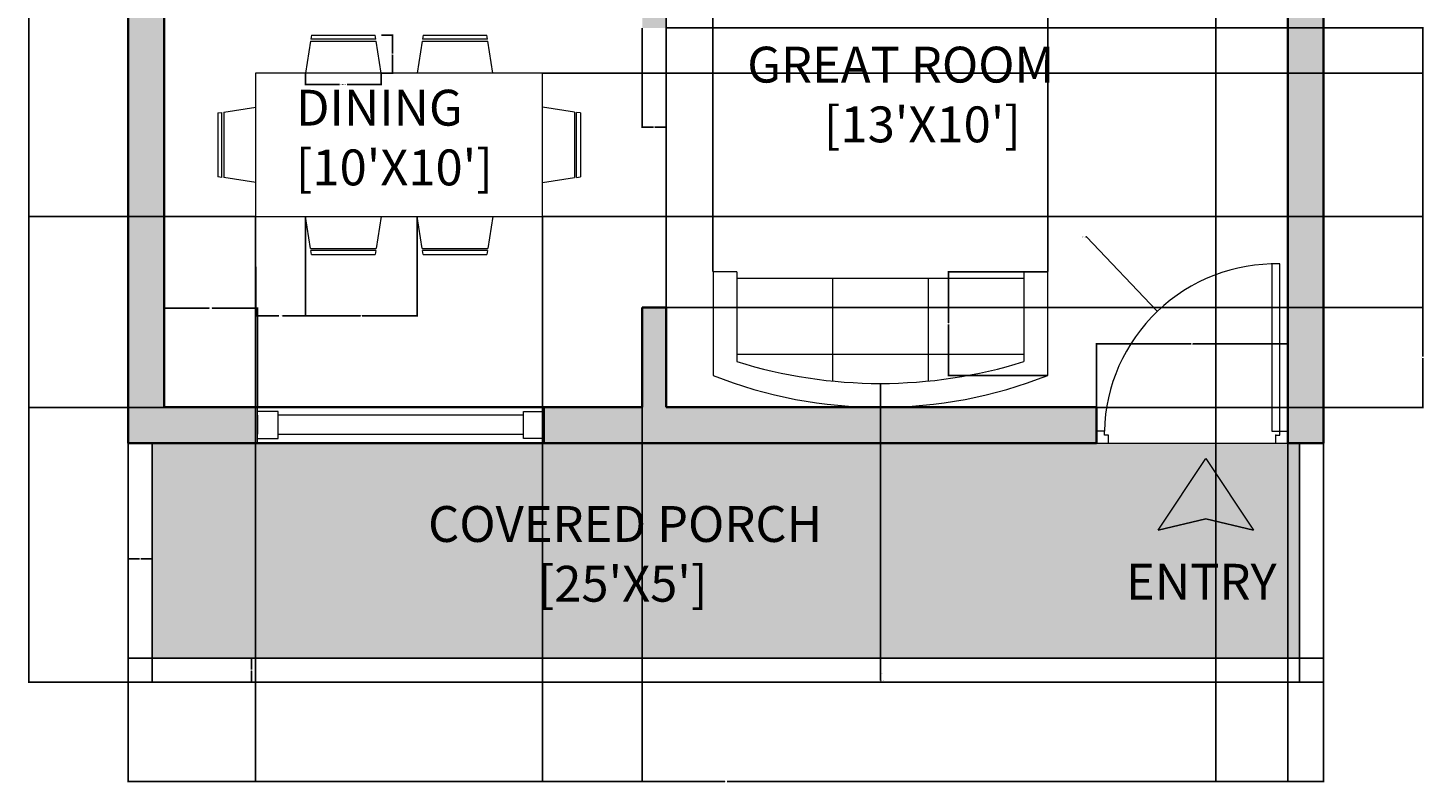
# Model space of a CAD drawing. Units: inches. Extents: x 2203 to 2554, y 381 to 929.
# Tile 1 of 3: x 2203 to 2554, y 381 to 570. Entities that reach past the tile are written whole.
import ezdxf

# ---------------------------------------------------------------- set-up
doc = ezdxf.new("R2010")
doc.units = ezdxf.units.IN
for name, color, linetype, lineweight in [('A-ANNO-DIMS', 2, 'Continuous', 18), ('A-ANNO-SYMB', 239, 'Continuous', 18), ('A-ANNO-TEXT', 7, 'Continuous', 18), ('A-AREA-IDEN', 7, 'Continuous', 18), ('A-DOOR', 239, 'Continuous', 18), ('A-FLOR', 7, 'Continuous', 25), ('A-FURN', 8, 'Continuous', 18), ('A-GLAZ', 4, 'Continuous', 18), ('A-WALL', 7, 'Continuous', 35), ('A-WALL-PATT', 250, 'Continuous', 13)]:
    doc.layers.add(name, color=color, linetype=linetype, lineweight=lineweight)
doc.layers.add('A-FLOR-PATT', color=241, linetype='Continuous', lineweight=13, true_color=0xf7abae)
doc.styles.get("Standard").update_dxf_attribs({"font": 'arial.ttf'})
doc.dimstyles.get("Standard").update_dxf_attribs({"dimtxt": 0.18, "dimasz": 0.18, "dimexe": 0.18, "dimexo": 0.0625, "dimgap": 0.09, "dimtad": 0, "dimtih": 1, "dimtoh": 1, "dimdec": 4, "dimzin": 0, "dimdsep": 46, "dimtxsty": 'Standard', "dimcen": 0.09, "dimadec": 0, "dimazin": 0, "dimtfac": 1, "dimtdec": 4, "dimtofl": 0, "dimtmove": 0, "dimatfit": 3, "dimfxl": 1, "dimtolj": 1, "dimtzin": 0, "dimarcsym": 0})

# ---------------------------------------------------------------- blocks, each defined once
blk = doc.blocks.new('WIN-72')
for p, q in [((0, 0), (0, 9)), ((0, 9), (72, 9)), ((5.2, 7.99), (0, 7.99)), ((5.2, 1.13), (5.2, 7.99)), ((66.8, 1.13), (66.8, 7.99)), ((66.8, 7.99), (72, 7.99)), ((72, 9), (72, 0)), ((72, 6.99), (72, 9)), ((0, 6.99), (0, 2.25)), ((0, 0), (0, 4.5)), ((66.8, 6.99), (5.2, 6.99)), ((72, 4.5), (72, 6.99)), ((72, 2.25), (72, 6.99)), ((0, 1.13), (5.2, 1.13)), ((72, 0), (0, 0)), ((5.2, 2.25), (66.8, 2.25)), ((72, 1.13), (66.8, 1.13)), ((72, 0), (72, 2.25))]:
    blk.add_line(p, q)
blk = doc.blocks.new('CHAIR-DINING')
for p, q in [((1.2504, 8.00297), (0, 0)), ((1.2543, 8.00238), (17.7239, 8.00238)), ((1.4847, 9.50238), (1.3285, 8.5028)), ((17.6431, 8.50238), (1.3313, 8.50238)), ((1.4847, 9.50238), (17.4847, 9.50238)), ((17.641, 8.50204), (17.4847, 9.50238)), ((18.9695, 0), (17.7192, 8.00164))]:
    blk.add_line(p, q)
blk = doc.blocks.new('*D13')
at = {"layer": 'A-ANNO-DIMS', "color": 0, "lineweight": -2, "transparency": 16777216}
for p, q in [((2273.11, 558.9), (2273.11, 555.94)), ((2292.08, 558.9), (2292.08, 555.94)), ((2273.29, 556.12), (2281.64, 556.12)), ((2291.9, 556.12), (2283.55, 556.12))]:
    blk.add_line(p, q, dxfattribs=at)
at = {"layer": 'A-ANNO-DIMS', "color": 0, "transparency": 16777216}
for points in [[(2273.29, 556.15), (2273.29, 556.09), (2273.11, 556.12)], [(2291.9, 556.15), (2291.9, 556.09), (2292.08, 556.12)]]:
    blk.add_solid(points, dxfattribs=at)
at = {"layer": 'Defpoints', "color": 0, "transparency": 16777216}
for p in [(2273.11, 558.96), (2292.08, 558.96), (2292.08, 556.12)]:
    blk.add_point(p, dxfattribs=at)
at = {"layer": 'A-ANNO-DIMS', "color": 0, "transparency": 16777216, "insert": (2282.59, 556.12), "char_height": 0.18, "attachment_point": 5}
blk.add_mtext('\\A1;CHAIR 19 TYP.', dxfattribs=at)
blk = doc.blocks.new('*D14')
at = {"layer": 'A-ANNO-DIMS', "color": 0, "lineweight": -2, "transparency": 16777216}
for p, q in [((2292.14, 568.47), (2295.1, 568.47)), ((2294.92, 568.29), (2294.92, 563.9)), ((2294.92, 559.14), (2294.92, 563.53)), ((2292.14, 558.96), (2295.1, 558.96))]:
    blk.add_line(p, q, dxfattribs=at)
at = {"layer": 'A-ANNO-DIMS', "color": 0, "transparency": 16777216}
for points in [[(2294.89, 568.29), (2294.95, 568.29), (2294.92, 568.47)], [(2294.89, 559.14), (2294.95, 559.14), (2294.92, 558.96)]]:
    blk.add_solid(points, dxfattribs=at)
at = {"layer": 'Defpoints', "color": 0, "transparency": 16777216}
for p in [(2292.08, 568.47), (2294.92, 568.47), (2292.08, 558.96)]:
    blk.add_point(p, dxfattribs=at)
at = {"layer": 'A-ANNO-DIMS', "color": 0, "transparency": 16777216, "insert": (2294.92, 563.71), "char_height": 0.18, "attachment_point": 5}
blk.add_mtext('\\A1;10 TYP.', dxfattribs=at)
blk = doc.blocks.new('*D21')
at = {"layer": 'A-ANNO-DIMS', "color": 0, "lineweight": -2, "transparency": 16777216}
for p, q in [((2228.6, 406), (2228.6, 380.96)), ((2528.6, 406), (2528.6, 380.96)), ((2228.78, 381.14), (2378.31, 381.14)), ((2528.42, 381.14), (2378.89, 381.14))]:
    blk.add_line(p, q, dxfattribs=at)
at = {"layer": 'A-ANNO-DIMS', "color": 0, "transparency": 16777216}
for points in [[(2228.78, 381.17), (2228.78, 381.11), (2228.6, 381.14)], [(2528.42, 381.17), (2528.42, 381.11), (2528.6, 381.14)]]:
    blk.add_solid(points, dxfattribs=at)
at = {"layer": 'Defpoints', "color": 0, "transparency": 16777216}
for p in [(2228.6, 406.06), (2528.6, 406.06), (2528.6, 381.14)]:
    blk.add_point(p, dxfattribs=at)
at = {"layer": 'A-ANNO-DIMS', "color": 0, "transparency": 16777216, "insert": (2378.6, 381.14), "char_height": 0.18, "attachment_point": 5}
blk.add_mtext('\\A1;300', dxfattribs=at)
blk = doc.blocks.new('*D22')
at = {"layer": 'A-ANNO-DIMS', "color": 0, "lineweight": -2, "transparency": 16777216}
for p, q in [((2228.54, 904.06), (2203.5, 904.06)), ((2203.68, 903.88), (2203.68, 655.25)), ((2203.68, 406.24), (2203.68, 654.88)), ((2228.54, 406.06), (2203.5, 406.06))]:
    blk.add_line(p, q, dxfattribs=at)
at = {"layer": 'A-ANNO-DIMS', "color": 0, "transparency": 16777216}
for points in [[(2203.65, 903.88), (2203.71, 903.88), (2203.68, 904.06)], [(2203.65, 406.24), (2203.71, 406.24), (2203.68, 406.06)]]:
    blk.add_solid(points, dxfattribs=at)
at = {"layer": 'Defpoints', "color": 0, "transparency": 16777216}
for p in [(2203.68, 904.06), (2228.6, 904.06), (2228.6, 406.06)]:
    blk.add_point(p, dxfattribs=at)
at = {"layer": 'A-ANNO-DIMS', "color": 0, "transparency": 16777216, "insert": (2203.68, 655.06), "char_height": 0.18, "attachment_point": 5}
blk.add_mtext('\\A1;498', dxfattribs=at)
blk = doc.blocks.new('*D25')
at = {"layer": 'A-ANNO-DIMS', "color": 0, "lineweight": -2, "transparency": 16777216}
for p, q in [((2237.6, 475.13), (2237.6, 500.16)), ((2237.78, 499.98), (2248.92, 499.98)), ((2260.85, 499.98), (2249.71, 499.98)), ((2261.03, 475.13), (2261.03, 500.16))]:
    blk.add_line(p, q, dxfattribs=at)
at = {"layer": 'A-ANNO-DIMS', "color": 0, "transparency": 16777216}
for points in [[(2237.78, 500.01), (2237.78, 499.95), (2237.6, 499.98)], [(2260.85, 500.01), (2260.85, 499.95), (2261.03, 499.98)]]:
    blk.add_solid(points, dxfattribs=at)
at = {"layer": 'Defpoints', "color": 0, "transparency": 16777216}
for p in [(2261.03, 499.98), (2237.6, 475.06), (2261.03, 475.06)]:
    blk.add_point(p, dxfattribs=at)
at = {"layer": 'A-ANNO-DIMS', "color": 0, "transparency": 16777216, "insert": (2249.31, 499.98), "char_height": 0.18, "attachment_point": 5}
blk.add_mtext('\\A1;23.43', dxfattribs=at)
blk = doc.blocks.new('*D28')
at = {"layer": 'A-ANNO-DIMS', "color": 0, "lineweight": -2, "transparency": 16777216}
for p, q in [((2357.6, 570.27), (2357.6, 545.23)), ((2363.6, 570.27), (2363.6, 545.23)), ((2357.78, 545.41), (2360.45, 545.41)), ((2363.42, 545.41), (2360.75, 545.41))]:
    blk.add_line(p, q, dxfattribs=at)
at = {"layer": 'A-ANNO-DIMS', "color": 0, "transparency": 16777216}
for points in [[(2357.78, 545.44), (2357.78, 545.38), (2357.6, 545.41)], [(2363.42, 545.44), (2363.42, 545.38), (2363.6, 545.41)]]:
    blk.add_solid(points, dxfattribs=at)
at = {"layer": 'Defpoints', "color": 0, "transparency": 16777216}
for p in [(2357.6, 570.33), (2363.6, 570.33), (2357.6, 545.41)]:
    blk.add_point(p, dxfattribs=at)
at = {"layer": 'A-ANNO-DIMS', "color": 0, "transparency": 16777216, "insert": (2360.6, 545.41), "char_height": 0.18, "attachment_point": 5}
blk.add_mtext('\\A1;6', dxfattribs=at)
blk = doc.blocks.new('*D32')
at = {"layer": 'A-ANNO-DIMS', "color": 0, "lineweight": -2, "transparency": 16777216}
for p, q in [((2363.66, 570.33), (2553.7, 570.33)), ((2553.52, 570.15), (2553.52, 535.42)), ((2553.52, 500.33), (2553.52, 535.06)), ((2363.66, 500.15), (2553.7, 500.15))]:
    blk.add_line(p, q, dxfattribs=at)
at = {"layer": 'A-ANNO-DIMS', "color": 0, "transparency": 16777216}
for points in [[(2553.49, 570.15), (2553.55, 570.15), (2553.52, 570.33)], [(2553.49, 500.33), (2553.55, 500.33), (2553.52, 500.15)]]:
    blk.add_solid(points, dxfattribs=at)
at = {"layer": 'Defpoints', "color": 0, "transparency": 16777216}
for p in [(2363.6, 570.33), (2553.52, 570.33), (2363.6, 500.15)]:
    blk.add_point(p, dxfattribs=at)
at = {"layer": 'A-ANNO-DIMS', "color": 0, "transparency": 16777216, "insert": (2553.52, 535.24), "char_height": 0.18, "attachment_point": 5}
blk.add_mtext('\\A1;70.18', dxfattribs=at)
blk = doc.blocks.new('*D33')
at = {"layer": 'A-ANNO-DIMS', "color": 0, "lineweight": -2, "transparency": 16777216}
for p, q in [((2363.66, 500.15), (2553.7, 500.15)), ((2553.52, 499.97), (2553.52, 487.79)), ((2553.52, 475.24), (2553.52, 487.42)), ((2363.66, 475.06), (2553.7, 475.06))]:
    blk.add_line(p, q, dxfattribs=at)
at = {"layer": 'A-ANNO-DIMS', "color": 0, "transparency": 16777216}
for points in [[(2553.49, 499.97), (2553.55, 499.97), (2553.52, 500.15)], [(2553.49, 475.24), (2553.55, 475.24), (2553.52, 475.06)]]:
    blk.add_solid(points, dxfattribs=at)
at = {"layer": 'Defpoints', "color": 0, "transparency": 16777216}
for p in [(2363.6, 500.15), (2553.52, 500.15), (2363.6, 475.06)]:
    blk.add_point(p, dxfattribs=at)
at = {"layer": 'A-ANNO-DIMS', "color": 0, "transparency": 16777216, "insert": (2553.52, 487.61), "char_height": 0.18, "attachment_point": 5}
blk.add_mtext('\\A1;25.08', dxfattribs=at)
blk = doc.blocks.new('*D34')
at = {"layer": 'A-ANNO-DIMS', "color": 0, "lineweight": -2, "transparency": 16777216}
for p, q in [((2471.6, 466.13), (2471.6, 491.16)), ((2471.78, 490.98), (2495.38, 490.98)), ((2519.42, 490.98), (2495.82, 490.98)), ((2519.6, 466.13), (2519.6, 491.16))]:
    blk.add_line(p, q, dxfattribs=at)
at = {"layer": 'A-ANNO-DIMS', "color": 0, "transparency": 16777216}
for points in [[(2471.78, 491.01), (2471.78, 490.95), (2471.6, 490.98)], [(2519.42, 491.01), (2519.42, 490.95), (2519.6, 490.98)]]:
    blk.add_solid(points, dxfattribs=at)
at = {"layer": 'Defpoints', "color": 0, "transparency": 16777216}
for p in [(2519.6, 490.98), (2471.6, 466.06), (2519.6, 466.06)]:
    blk.add_point(p, dxfattribs=at)
at = {"layer": 'A-ANNO-DIMS', "color": 0, "transparency": 16777216, "insert": (2495.6, 490.98), "char_height": 0.18, "attachment_point": 5}
blk.add_mtext('\\A1;48', dxfattribs=at)
blk = doc.blocks.new('*D41')
at = {"layer": 'A-ANNO-DIMS', "color": 0, "lineweight": -2, "transparency": 16777216}
for p, q in [((2375.37, 509.13), (2375.37, 929.16)), ((2375.55, 928.98), (2417.15, 928.98)), ((2459.19, 928.98), (2417.59, 928.98)), ((2459.37, 509.13), (2459.37, 929.16))]:
    blk.add_line(p, q, dxfattribs=at)
at = {"layer": 'A-ANNO-DIMS', "color": 0, "transparency": 16777216}
for points in [[(2375.55, 929.01), (2375.55, 928.95), (2375.37, 928.98)], [(2459.19, 929.01), (2459.19, 928.95), (2459.37, 928.98)]]:
    blk.add_solid(points, dxfattribs=at)
at = {"layer": 'Defpoints', "color": 0, "transparency": 16777216}
for p in [(2459.37, 928.98), (2375.37, 509.06), (2459.37, 509.06)]:
    blk.add_point(p, dxfattribs=at)
at = {"layer": 'A-ANNO-DIMS', "color": 0, "transparency": 16777216, "insert": (2417.37, 928.98), "char_height": 0.18, "attachment_point": 5}
blk.add_mtext('\\A1;84', dxfattribs=at)
blk = doc.blocks.new('*D42')
at = {"layer": 'A-ANNO-DIMS', "color": 0, "lineweight": -2, "transparency": 16777216}
for p, q in [((2459.31, 509.06), (2434.27, 509.06)), ((2434.45, 508.88), (2434.45, 496.25)), ((2434.45, 483.24), (2434.45, 495.88)), ((2459.31, 483.06), (2434.27, 483.06))]:
    blk.add_line(p, q, dxfattribs=at)
at = {"layer": 'A-ANNO-DIMS', "color": 0, "transparency": 16777216}
for points in [[(2434.42, 508.88), (2434.48, 508.88), (2434.45, 509.06)], [(2434.42, 483.24), (2434.48, 483.24), (2434.45, 483.06)]]:
    blk.add_solid(points, dxfattribs=at)
at = {"layer": 'Defpoints', "color": 0, "transparency": 16777216}
for p in [(2434.45, 509.06), (2459.37, 509.06), (2459.37, 483.06)]:
    blk.add_point(p, dxfattribs=at)
at = {"layer": 'A-ANNO-DIMS', "color": 0, "transparency": 16777216, "insert": (2434.45, 496.06), "char_height": 0.18, "attachment_point": 5}
blk.add_mtext('\\A1;26', dxfattribs=at)
blk = doc.blocks.new('*D43')
at = {"layer": 'A-ANNO-DIMS', "color": 0, "lineweight": -2, "transparency": 16777216}
for p, q in [((2363.6, 500.21), (2363.6, 929.16)), ((2363.78, 928.98), (2369.03, 928.98)), ((2375.19, 928.98), (2369.94, 928.98)), ((2375.37, 509.13), (2375.37, 929.16))]:
    blk.add_line(p, q, dxfattribs=at)
at = {"layer": 'A-ANNO-DIMS', "color": 0, "transparency": 16777216}
for points in [[(2363.78, 929.01), (2363.78, 928.95), (2363.6, 928.98)], [(2375.19, 929.01), (2375.19, 928.95), (2375.37, 928.98)]]:
    blk.add_solid(points, dxfattribs=at)
at = {"layer": 'Defpoints', "color": 0, "transparency": 16777216}
for p in [(2375.37, 928.98), (2375.37, 509.06), (2363.6, 500.15)]:
    blk.add_point(p, dxfattribs=at)
at = {"layer": 'A-ANNO-DIMS', "color": 0, "transparency": 16777216, "insert": (2369.49, 928.98), "char_height": 0.18, "attachment_point": 5}
blk.add_mtext('\\A1;11.775', dxfattribs=at)
blk = doc.blocks.new('*D44')
at = {"layer": 'A-ANNO-DIMS', "color": 0, "lineweight": -2, "transparency": 16777216}
for p, q in [((2260.59, 522.9), (2260.59, 380.96)), ((2332.59, 522.9), (2332.59, 380.96)), ((2260.77, 381.14), (2296.38, 381.14)), ((2332.41, 381.14), (2296.81, 381.14))]:
    blk.add_line(p, q, dxfattribs=at)
at = {"layer": 'A-ANNO-DIMS', "color": 0, "transparency": 16777216}
for points in [[(2260.77, 381.17), (2260.77, 381.11), (2260.59, 381.14)], [(2332.41, 381.17), (2332.41, 381.11), (2332.59, 381.14)]]:
    blk.add_solid(points, dxfattribs=at)
at = {"layer": 'Defpoints', "color": 0, "transparency": 16777216}
for p in [(2260.59, 522.97), (2332.59, 522.97), (2332.59, 381.14)]:
    blk.add_point(p, dxfattribs=at)
at = {"layer": 'A-ANNO-DIMS', "color": 0, "transparency": 16777216, "insert": (2296.59, 381.14), "char_height": 0.18, "attachment_point": 5}
blk.add_mtext('\\A1;72', dxfattribs=at)
blk = doc.blocks.new('*D45')
at = {"layer": 'A-ANNO-DIMS', "color": 0, "lineweight": -2, "transparency": 16777216}
for p, q in [((2332.66, 558.97), (2553.7, 558.97)), ((2553.52, 558.79), (2553.52, 541.15)), ((2553.52, 523.15), (2553.52, 540.78)), ((2332.66, 522.97), (2553.7, 522.97))]:
    blk.add_line(p, q, dxfattribs=at)
at = {"layer": 'A-ANNO-DIMS', "color": 0, "transparency": 16777216}
for points in [[(2553.49, 558.79), (2553.55, 558.79), (2553.52, 558.97)], [(2553.49, 523.15), (2553.55, 523.15), (2553.52, 522.97)]]:
    blk.add_solid(points, dxfattribs=at)
at = {"layer": 'Defpoints', "color": 0, "transparency": 16777216}
for p in [(2332.59, 558.97), (2332.59, 522.97), (2553.52, 522.97)]:
    blk.add_point(p, dxfattribs=at)
at = {"layer": 'A-ANNO-DIMS', "color": 0, "transparency": 16777216, "insert": (2553.52, 540.97), "char_height": 0.18, "attachment_point": 5}
blk.add_mtext('\\A1;36', dxfattribs=at)
blk = doc.blocks.new('*D46')
at = {"layer": 'A-ANNO-DIMS', "color": 0, "lineweight": -2, "transparency": 16777216}
for p, q in [((2332.59, 522.9), (2332.59, 380.96)), ((2357.6, 500.08), (2357.6, 380.96)), ((2332.77, 381.14), (2344.63, 381.14)), ((2357.42, 381.14), (2345.56, 381.14))]:
    blk.add_line(p, q, dxfattribs=at)
at = {"layer": 'A-ANNO-DIMS', "color": 0, "transparency": 16777216}
for points in [[(2332.77, 381.17), (2332.77, 381.11), (2332.59, 381.14)], [(2357.42, 381.17), (2357.42, 381.11), (2357.6, 381.14)]]:
    blk.add_solid(points, dxfattribs=at)
at = {"layer": 'Defpoints', "color": 0, "transparency": 16777216}
for p in [(2332.59, 522.97), (2357.6, 500.15), (2357.6, 381.14)]:
    blk.add_point(p, dxfattribs=at)
at = {"layer": 'A-ANNO-DIMS', "color": 0, "transparency": 16777216, "insert": (2345.1, 381.14), "char_height": 0.18, "attachment_point": 5}
blk.add_mtext('\\A1;25.004', dxfattribs=at)
blk = doc.blocks.new('*D47')
at = {"layer": 'A-ANNO-DIMS', "color": 0, "lineweight": -2, "transparency": 16777216}
for p, q in [((2260.53, 522.97), (2203.5, 522.97)), ((2203.68, 522.79), (2203.68, 499.2)), ((2203.68, 475.24), (2203.68, 498.83)), ((2237.54, 475.06), (2203.5, 475.06))]:
    blk.add_line(p, q, dxfattribs=at)
at = {"layer": 'A-ANNO-DIMS', "color": 0, "transparency": 16777216}
for points in [[(2203.65, 522.79), (2203.71, 522.79), (2203.68, 522.97)], [(2203.65, 475.24), (2203.71, 475.24), (2203.68, 475.06)]]:
    blk.add_solid(points, dxfattribs=at)
at = {"layer": 'Defpoints', "color": 0, "transparency": 16777216}
for p in [(2260.59, 522.97), (2203.68, 475.06), (2237.6, 475.06)]:
    blk.add_point(p, dxfattribs=at)
at = {"layer": 'A-ANNO-DIMS', "color": 0, "transparency": 16777216, "insert": (2203.68, 499.02), "char_height": 0.18, "attachment_point": 5}
blk.add_mtext('\\A1;47.9', dxfattribs=at)
blk = doc.blocks.new('*D48')
at = {"layer": 'A-ANNO-DIMS', "color": 0, "lineweight": -2, "transparency": 16777216}
for p, q in [((2260.59, 522.9), (2260.6, 497.87)), ((2273.11, 522.91), (2273.11, 497.87)), ((2260.78, 498.05), (2266.4, 498.05)), ((2272.93, 498.05), (2267.31, 498.05))]:
    blk.add_line(p, q, dxfattribs=at)
at = {"layer": 'A-ANNO-DIMS', "color": 0, "transparency": 16777216}
for points in [[(2260.78, 498.08), (2260.78, 498.02), (2260.6, 498.05)], [(2272.93, 498.08), (2272.93, 498.02), (2273.11, 498.05)]]:
    blk.add_solid(points, dxfattribs=at)
at = {"layer": 'Defpoints', "color": 0, "transparency": 16777216}
for p in [(2260.59, 522.97), (2273.11, 522.97), (2260.6, 498.05)]:
    blk.add_point(p, dxfattribs=at)
at = {"layer": 'A-ANNO-DIMS', "color": 0, "transparency": 16777216, "insert": (2266.86, 498.05), "char_height": 0.18, "attachment_point": 5}
blk.add_mtext('\\A1;12.515', dxfattribs=at)
blk = doc.blocks.new('*D49')
at = {"layer": 'A-ANNO-DIMS', "color": 0, "lineweight": -2, "transparency": 16777216}
for p, q in [((2273.11, 522.91), (2273.11, 497.87)), ((2301.11, 522.91), (2301.11, 497.87)), ((2273.29, 498.05), (2286.89, 498.05)), ((2300.93, 498.05), (2287.33, 498.05))]:
    blk.add_line(p, q, dxfattribs=at)
at = {"layer": 'A-ANNO-DIMS', "color": 0, "transparency": 16777216}
for points in [[(2273.29, 498.08), (2273.29, 498.02), (2273.11, 498.05)], [(2300.93, 498.08), (2300.93, 498.02), (2301.11, 498.05)]]:
    blk.add_solid(points, dxfattribs=at)
at = {"layer": 'Defpoints', "color": 0, "transparency": 16777216}
for p in [(2273.11, 522.97), (2301.11, 522.97), (2273.11, 498.05)]:
    blk.add_point(p, dxfattribs=at)
at = {"layer": 'A-ANNO-DIMS', "color": 0, "transparency": 16777216, "insert": (2287.11, 498.05), "char_height": 0.18, "attachment_point": 5}
blk.add_mtext('\\A1;28', dxfattribs=at)
blk = doc.blocks.new('*D55')
at = {"layer": 'A-ANNO-DIMS', "color": 0, "lineweight": -2, "transparency": 16777216}
for p, q in [((2501.6, 739.61), (2501.6, 380.96)), ((2519.6, 727), (2519.6, 380.96)), ((2501.78, 381.14), (2510.39, 381.14)), ((2519.42, 381.14), (2510.81, 381.14))]:
    blk.add_line(p, q, dxfattribs=at)
at = {"layer": 'A-ANNO-DIMS', "color": 0, "transparency": 16777216}
for points in [[(2501.78, 381.17), (2501.78, 381.11), (2501.6, 381.14)], [(2519.42, 381.17), (2519.42, 381.11), (2519.6, 381.14)]]:
    blk.add_solid(points, dxfattribs=at)
at = {"layer": 'Defpoints', "color": 0, "transparency": 16777216}
for p in [(2501.6, 739.68), (2519.6, 727.06), (2519.6, 381.14)]:
    blk.add_point(p, dxfattribs=at)
at = {"layer": 'A-ANNO-DIMS', "color": 0, "transparency": 16777216, "insert": (2510.6, 381.14), "char_height": 0.18, "attachment_point": 5}
blk.add_mtext('\\A1;18', dxfattribs=at)
blk = doc.blocks.new('*D56')
at = {"layer": 'A-ANNO-DIMS', "color": 0, "lineweight": -2, "transparency": 16777216}
for p, q in [((2234.66, 412.06), (2259.7, 412.06)), ((2259.52, 411.88), (2259.52, 409.25)), ((2259.52, 406.24), (2259.52, 408.88)), ((2234.66, 406.06), (2259.7, 406.06))]:
    blk.add_line(p, q, dxfattribs=at)
at = {"layer": 'A-ANNO-DIMS', "color": 0, "transparency": 16777216}
for points in [[(2259.49, 411.88), (2259.55, 411.88), (2259.52, 412.06)], [(2259.49, 406.24), (2259.55, 406.24), (2259.52, 406.06)]]:
    blk.add_solid(points, dxfattribs=at)
at = {"layer": 'Defpoints', "color": 0, "transparency": 16777216}
for p in [(2234.6, 412.06), (2234.6, 406.06), (2259.52, 406.06)]:
    blk.add_point(p, dxfattribs=at)
at = {"layer": 'A-ANNO-DIMS', "color": 0, "transparency": 16777216, "insert": (2259.52, 409.06), "char_height": 0.18, "attachment_point": 5}
blk.add_mtext('\\A1;6', dxfattribs=at)
blk = doc.blocks.new('*D57')
at = {"layer": 'A-ANNO-DIMS', "color": 0, "lineweight": -2, "transparency": 16777216}
for p, q in [((2228.6, 412.13), (2228.6, 437.16)), ((2228.78, 436.98), (2231.45, 436.98)), ((2234.42, 436.98), (2231.75, 436.98)), ((2234.6, 412.13), (2234.6, 437.16))]:
    blk.add_line(p, q, dxfattribs=at)
at = {"layer": 'A-ANNO-DIMS', "color": 0, "transparency": 16777216}
for points in [[(2228.78, 437.01), (2228.78, 436.95), (2228.6, 436.98)], [(2234.42, 437.01), (2234.42, 436.95), (2234.6, 436.98)]]:
    blk.add_solid(points, dxfattribs=at)
at = {"layer": 'Defpoints', "color": 0, "transparency": 16777216}
for p in [(2234.6, 436.98), (2228.6, 412.06), (2234.6, 412.06)]:
    blk.add_point(p, dxfattribs=at)
at = {"layer": 'A-ANNO-DIMS', "color": 0, "transparency": 16777216, "insert": (2231.6, 436.98), "char_height": 0.18, "attachment_point": 5}
blk.add_mtext('\\A1;6', dxfattribs=at)
blk = doc.blocks.new('*D60')
at = {"layer": 'A-ANNO-DIMS', "color": 0, "lineweight": -2, "transparency": 16777216}
for p, q in [((2417.28, 602.26), (2417.46, 602.26)), ((2417.37, 602.17), (2417.37, 602.35)), ((2417.37, 408.35), (2417.37, 480.88)), ((2417.55, 408.35), (2417.37, 408.35))]:
    blk.add_line(p, q, dxfattribs=at)
at = {"layer": 'A-ANNO-DIMS', "color": 0, "transparency": 16777216}
blk.add_solid([(2417.4, 480.88), (2417.34, 480.88), (2417.37, 481.06)], dxfattribs=at)
at = {"layer": 'Defpoints', "color": 0, "transparency": 16777216}
for p in [(2417.37, 602.26), (2417.37, 481.06)]:
    blk.add_point(p, dxfattribs=at)
at = {"layer": 'A-ANNO-DIMS', "color": 0, "transparency": 16777216, "insert": (2418.03, 408.35), "char_height": 0.18, "attachment_point": 5}
blk.add_mtext('\\A1;R121.2', dxfattribs=at)
blk = doc.blocks.new('*D61')
at = {"layer": 'A-ANNO-DIMS', "color": 0, "lineweight": -2, "transparency": 16777216}
for p, q in [((2417.28, 589.31), (2417.46, 589.31)), ((2417.37, 589.22), (2417.37, 589.4)), ((2417.37, 406.51), (2417.37, 474.88)), ((2417.55, 406.51), (2417.37, 406.51))]:
    blk.add_line(p, q, dxfattribs=at)
at = {"layer": 'A-ANNO-DIMS', "color": 0, "transparency": 16777216}
blk.add_solid([(2417.4, 474.88), (2417.34, 474.88), (2417.37, 475.06)], dxfattribs=at)
at = {"layer": 'Defpoints', "color": 0, "transparency": 16777216}
for p in [(2417.37, 589.31), (2417.37, 475.06)]:
    blk.add_point(p, dxfattribs=at)
at = {"layer": 'A-ANNO-DIMS', "color": 0, "transparency": 16777216, "insert": (2418.1, 406.51), "char_height": 0.18, "attachment_point": 5}
blk.add_mtext('\\A1;R114.25', dxfattribs=at)
blk = doc.blocks.new('*D62')
at = {"layer": 'A-ANNO-DIMS', "color": 0, "lineweight": -2, "transparency": 16777216}
for p, q in [((2468.9, 517.85), (2469.08, 517.85)), ((2469.08, 517.85), (2486.78, 499.31)), ((2516.51, 468.06), (2516.69, 468.06)), ((2516.6, 467.97), (2516.6, 468.15))]:
    blk.add_line(p, q, dxfattribs=at)
at = {"layer": 'A-ANNO-DIMS', "color": 0, "transparency": 16777216}
blk.add_solid([(2486.8, 499.33), (2486.75, 499.29), (2486.9, 499.18)], dxfattribs=at)
at = {"layer": 'Defpoints', "color": 0, "transparency": 16777216}
for p in [(2486.9, 499.18), (2516.6, 468.06)]:
    blk.add_point(p, dxfattribs=at)
at = {"layer": 'A-ANNO-DIMS', "color": 0, "transparency": 16777216, "insert": (2468.44, 517.85), "char_height": 0.18, "attachment_point": 5}
blk.add_mtext('\\A1;R43.01', dxfattribs=at)

msp = doc.modelspace()

# ---------------------------------------------------------------- hatches: boundary and pattern name
at = {"layer": 'A-ANNO-SYMB', "transparency": 33554457}
h = msp.add_hatch(color=256, dxfattribs=at)
h.dxf.hatch_style = 1
h.paths.add_polyline_path([(2499.0485, 462.247), (2487.1138, 444.2048), (2499.0313, 447.0534), (2510.9832, 444.2048)])
at = {"layer": 'A-FLOR-PATT', "transparency": 33554582}
h = msp.add_hatch(color=256, dxfattribs=at)
h.dxf.hatch_style = 1
h.paths.add_polyline_path([(2522.599, 466.0647), (2519.599, 466.0647), (2471.599, 466.0647), (2234.599, 466.0647), (2234.599, 412.0647), (2522.599, 412.0647)])
h.paths.add_polyline_path([(2487.1138, 444.2048), (2499.0485, 462.247), (2510.9832, 444.2048), (2499.0313, 447.0534)], flags=16)
h.paths.add_polyline_path([(2475.782, 421.8559), (2522.8939, 421.8559), (2522.8939, 440.4023), (2475.782, 440.4023)], flags=9)
h.paths.add_polyline_path([(2300.9929, 421.1579), (2416.5686, 421.1579), (2416.5686, 454.7412), (2300.9929, 454.7412)], flags=24)
h = msp.add_hatch(color=256, dxfattribs=at)
h.dxf.hatch_style = 1
h.paths.add_polyline_path([(2522.599, 466.0647), (2519.599, 466.0647), (2471.599, 466.0647), (2234.599, 466.0647), (2234.599, 412.0647), (2522.599, 412.0647)])
h.paths.add_polyline_path([(2487.1138, 444.2048), (2499.0485, 462.247), (2510.9832, 444.2048), (2499.0313, 447.0534)], flags=16)
h.paths.add_polyline_path([(2475.782, 421.8559), (2522.8939, 421.8559), (2522.8939, 440.4023), (2475.782, 440.4023)], flags=9)
h.paths.add_polyline_path([(2300.9929, 421.1579), (2416.5686, 421.1579), (2416.5686, 454.7412), (2300.9929, 454.7412)], flags=24)
at = {"layer": 'A-WALL-PATT'}
h = msp.add_hatch(color=256, dxfattribs=at)
h.dxf.hatch_style = 1
h.paths.add_polyline_path([(2237.599, 595.0647), (2260.3281, 595.0647), (2260.3281, 601.0647), (2237.599, 601.0647), (2237.599, 621.2584), (2233.099, 621.2584), (2230.6109, 621.2584), (2228.599, 621.2584), (2228.599, 466.0647), (2261.0302, 466.0647), (2261.0302, 470.5647), (2261.0302, 473.0528), (2261.0302, 475.0647), (2237.599, 475.0647)])
h.paths.add_polyline_path([(2237.599, 895.0647), (2305.0273, 895.0647), (2305.0273, 899.5647), (2305.0273, 904.0647), (2228.599, 904.0647), (2228.599, 693.2584), (2230.6109, 693.2584), (2235.349, 693.2584), (2237.599, 693.2584), (2237.599, 721.2436), (2357.599, 721.2436), (2357.599, 601.0647), (2331.8237, 601.0647), (2331.8237, 595.0647), (2357.599, 595.0647), (2357.599, 570.3283), (2363.599, 570.3283), (2363.599, 595.0647), (2363.599, 601.0647), (2363.599, 721.2436), (2399.5308, 721.2436), (2399.5308, 724.2436), (2399.5308, 727.0647), (2237.599, 727.0647)])
h.paths.add_polyline_path([(2447.599, 859.3877), (2441.8244, 859.3877), (2441.8244, 727.0647), (2441.8244, 721.2436), (2441.8244, 691.5632), (2441.8244, 631.1686), (2444.8244, 631.1686), (2447.599, 631.1686), (2447.599, 721.2436), (2519.599, 721.2436), (2519.599, 691.5572), (2524.099, 691.5572), (2526.3564, 691.5572), (2528.599, 691.5572), (2528.599, 904.0647), (2496.9662, 904.0647), (2496.9662, 901.8221), (2496.9662, 895.0647), (2519.599, 895.0647), (2519.599, 727.0647), (2447.599, 727.0647)])
h.paths.add_polyline_path([(2460.78, 904.0647), (2377.0273, 904.0647), (2377.0273, 902.0528), (2377.0273, 895.0647), (2441.8244, 895.0647), (2460.78, 895.0647), (2460.78, 899.5647)])
h.paths.add_polyline_path([(2471.599, 475.0647), (2363.599, 475.0647), (2363.599, 500.1465), (2357.599, 500.1465), (2357.599, 475.0647), (2333.0302, 475.0647), (2333.0302, 473.0528), (2333.0302, 468.3147), (2333.0302, 466.0647), (2471.599, 466.0647), (2471.599, 469.0647)])
h = msp.add_hatch(color=256, dxfattribs=at)
h.dxf.hatch_style = 1
h.paths.add_polyline_path([(2528.599, 655.371), (2526.3564, 655.371), (2519.599, 655.371), (2519.599, 601.0647), (2441.8244, 601.0647), (2441.8244, 595.0647), (2519.599, 595.0647), (2519.599, 475.0647), (2519.599, 466.0647), (2528.599, 466.0647)])

# ---------------------------------------------------------------- linework, layer by layer
at = {"layer": 'A-ANNO-SYMB'}
for p, q in [((2487.1138, 444.2048), (2499.0485, 462.247)), ((2487.1138, 444.2048), (2499.0485, 462.247)), ((2499.0485, 462.247), (2510.9832, 444.2048)), ((2499.0485, 462.247), (2510.9832, 444.2048)), ((2487.1138, 444.2048), (2499.0313, 447.0534)), ((2499.0313, 447.0534), (2487.1138, 444.2048)), ((2499.0313, 447.0534), (2510.9832, 444.2048)), ((2510.9832, 444.2048), (2499.0313, 447.0534))]:
    msp.add_line(p, q, dxfattribs=at)
at = {"layer": 'A-DOOR'}
for p, q in [((2517.599, 511.0647), (2515.599, 511.0647)), ((2515.599, 511.0647), (2515.599, 469.0647)), ((2517.599, 469.0647), (2517.599, 511.0647)), ((2471.599, 469.0647), (2471.599, 466.0647)), ((2473.599, 469.0647), (2471.599, 469.0647)), ((2471.599, 466.0647), (2474.599, 466.0647)), ((2471.599, 466.0647), (2474.599, 466.0647)), ((2471.599, 466.0647), (2519.599, 466.0647)), ((2473.599, 468.0647), (2473.599, 469.0647)), ((2474.599, 468.0647), (2473.599, 468.0647)), ((2474.599, 466.0647), (2474.599, 468.0647)), ((2515.599, 469.0647), (2517.599, 469.0647)), ((2516.599, 466.0647), (2516.599, 468.0647)), ((2516.599, 468.0647), (2517.599, 468.0647)), ((2516.599, 466.0647), (2519.599, 466.0647)), ((2517.599, 468.0647), (2517.599, 469.0647)), ((2517.599, 469.0647), (2519.599, 469.0647)), ((2519.599, 469.0647), (2519.599, 466.0647))]:
    msp.add_line(p, q, dxfattribs=at)
msp.add_arc((2516.599, 468.0647), 43.0116, 88.66778, 178.66778, dxfattribs=at)
at = {"layer": 'A-FLOR'}
for p, q in [((2468.599, 466.0647), (2228.599, 466.0647)), ((2228.599, 466.0647), (2228.599, 406.0647)), ((2234.599, 466.0647), (2234.599, 412.0647)), ((2522.599, 412.0647), (2522.599, 466.0647)), ((2528.599, 466.0647), (2522.599, 466.0647)), ((2528.599, 406.0647), (2528.599, 466.0647)), ((2528.599, 412.0647), (2228.599, 412.0647)), ((2234.599, 412.0647), (2234.599, 406.0647)), ((2234.599, 412.0647), (2462.599, 412.0647)), ((2462.599, 412.0647), (2468.599, 412.0647)), ((2522.599, 406.0647), (2522.599, 412.0647)), ((2228.599, 406.0647), (2528.599, 406.0647))]:
    msp.add_line(p, q, dxfattribs=at)
at = {"layer": 'A-FURN'}
for p, q in [((2332.5947, 558.9661), (2260.5947, 558.9661)), ((2260.5947, 558.9661), (2260.5947, 522.9661)), ((2332.5947, 522.9661), (2332.5947, 558.9661)), ((2260.5947, 522.9661), (2332.5947, 522.9661)), ((2381.3736, 509.0647), (2381.3736, 486.5343)), ((2453.3736, 509.0647), (2453.3736, 486.5343)), ((2381.3736, 507.5068), (2453.3736, 507.5068)), ((2405.3736, 507.5068), (2405.3736, 481.6618)), ((2429.3736, 507.5068), (2429.3736, 481.6618)), ((2381.3738, 488.4466), (2453.3735, 488.4466))]:
    msp.add_line(p, q, dxfattribs=at)
for points in [[(2381.3736, 509.0647), (2375.3736, 509.0647), (2375.3736, 483.0647)], [(2459.3736, 483.0647), (2459.3736, 509.0647), (2453.3736, 509.0647)]]:
    msp.add_lwpolyline(points, dxfattribs=at)
for centre, radius, start, end in [((2417.3736, 602.2615), 121.1968, 252.7203, 287.27967), ((2417.3737, 589.3147), 114.25, 248.4314, 291.56859)]:
    msp.add_arc(centre, radius, start, end, dxfattribs=at)
at = {"layer": 'A-WALL'}
for p, q in [((2228.599, 466.0647), (2228.599, 904.0647)), ((2528.599, 904.0647), (2528.599, 466.0647)), ((2528.599, 466.0647), (2528.599, 904.0647)), ((2237.599, 475.0647), (2237.599, 595.0647)), ((2519.599, 595.0647), (2519.599, 475.0647)), ((2357.599, 475.0647), (2357.599, 500.1465)), ((2357.599, 500.1465), (2363.599, 500.1465)), ((2363.599, 475.0647), (2363.599, 500.1465)), ((2237.599, 475.0647), (2357.599, 475.0647)), ((2357.599, 475.0647), (2237.599, 475.0647)), ((2471.1483, 475.0647), (2363.599, 475.0647)), ((2471.599, 475.0647), (2363.599, 475.0647)), ((2471.599, 466.0647), (2471.599, 475.0647)), ((2519.599, 475.0647), (2519.599, 466.0647)), ((2228.599, 466.0647), (2471.599, 466.0647)), ((2528.599, 466.0647), (2519.599, 466.0647)), ((2519.599, 466.0647), (2528.599, 466.0647))]:
    msp.add_line(p, q, dxfattribs=at)

# ---------------------------------------------------------------- block references
at = {"layer": 'A-FURN'}
for p in [(2273.11, 558.9637), (2301.11, 558.9637)]:
    msp.add_blockref('CHAIR-DINING', p, dxfattribs=at)
at = {"layer": 'A-FURN', "extrusion": (0, 0, -1), "zscale": -1}
for p, rotation in [((-2260.597, 550.4508), 270), ((-2273.11, 522.9685), 180), ((-2301.11, 522.9685), 180)]:
    msp.add_blockref('CHAIR-DINING', p, dxfattribs=dict(at, rotation=rotation))
at = {"layer": 'A-FURN', "rotation": 270}
msp.add_blockref('CHAIR-DINING', (2332.5923, 550.4508), dxfattribs=at)
at = {"layer": 'A-GLAZ'}
msp.add_blockref('WIN-72', (2261.0302, 466.0647), dxfattribs=at)

# ---------------------------------------------------------------- texts
at = {"layer": 'A-ANNO-TEXT', "insert": (2479.0266, 435.7703), "char_height": 9, "attachment_point": 1}
msp.add_mtext_dynamic_manual_height_columns('ENTRY', width=48.465527, gutter_width=12.5, heights=[13.2337], dxfattribs=at)
at = {"layer": 'A-AREA-IDEN', "char_height": 9, "attachment_point": 1}
for s, width, insert in [("GREAT ROOM\\P       [13'X10']", 95.127561, (2383.9648, 565.609)), ("DINING\\P[10'X10']", 83.503544, (2270.6925, 554.7972)), ("COVERED PORCH\\P          [25'X5']", 116.067637, (2303.8691, 450.2688))]:
    msp.add_mtext_dynamic_manual_height_columns(s, width=width, gutter_width=12.5, heights=[0], dxfattribs=dict(at, insert=insert))

# ---------------------------------------------------------------- dimensions: what is measured, and where the dimension line sits
at = {"layer": 'A-ANNO-DIMS'}
for base, p1, p2, override, picture, middle in [((2375.3736, 928.9847), (2363.599, 500.1465), (2375.3736, 509.0647), {"dimdec": 3, "dimlfac": 1, "dimrnd": 0, "dimzin": 0, "dimdsep": 46, "dimlunit": 2}, '*D43', (2369.4863, 928.9847)), ((2459.3736, 928.9847), (2375.3736, 509.0647), (2459.3736, 509.0647), {"dimdec": 0, "dimlfac": 1, "dimrnd": 0, "dimzin": 0, "dimdsep": 46, "dimlunit": 2}, '*D41', (2417.3736, 928.9847)), ((2519.599, 381.1447), (2501.599, 739.6759), (2519.599, 727.0647), {"dimdec": 0, "dimlfac": 1, "dimrnd": 0, "dimzin": 0, "dimdsep": 46, "dimlunit": 2}, '*D55', (2510.599, 381.1447)), ((2332.5947, 381.1447), (2260.5947, 522.9661), (2332.5947, 522.9661), {"dimdec": 0, "dimlfac": 1, "dimrnd": 0, "dimzin": 0, "dimdsep": 46, "dimlunit": 2}, '*D44', (2296.5947, 381.1447)), ((2357.599, 381.1447), (2332.5947, 522.9661), (2357.599, 500.1465), {"dimdec": 3, "dimlfac": 1, "dimrnd": 0, "dimzin": 0, "dimdsep": 46, "dimlunit": 2}, '*D46', (2345.0968, 381.1447)), ((2234.599, 436.9847), (2228.599, 412.0647), (2234.599, 412.0647), {"dimdec": 0, "dimlfac": 1, "dimrnd": 0, "dimzin": 0, "dimdsep": 46, "dimlunit": 2}, '*D57', (2231.599, 436.9847)), ((2528.599, 381.1447), (2228.599, 406.0647), (2528.599, 406.0647), {"dimdec": 0, "dimlfac": 1, "dimrnd": 0, "dimzin": 0, "dimdsep": 46, "dimlunit": 2}, '*D21', (2378.599, 381.1447))]:
    dim = msp.add_linear_dim(base=base, p1=p1, p2=p2, dimstyle='Standard', override=override, dxfattribs=at)
    dim.commit()
    dim.dimension.update_dxf_attribs({"geometry": picture, "text_midpoint": middle})
for base, p1, p2, angle, override, picture, middle in [((2203.679, 904.0647), (2228.599, 406.0647), (2228.599, 904.0647), 90, {"dimdec": 0, "dimlfac": 1, "dimrnd": 0, "dimzin": 0, "dimdsep": 46, "dimlunit": 2}, '*D22', (2203.679, 655.0647)), ((2357.599, 545.4083), (2363.599, 570.3283), (2357.599, 570.3283), 180, {"dimdec": 0, "dimlfac": 1, "dimrnd": 0, "dimzin": 0, "dimdsep": 46, "dimlunit": 2}, '*D28', (2360.599, 545.4083)), ((2553.519, 570.3283), (2363.599, 500.1465), (2363.599, 570.3283), 90, {"dimdec": 2, "dimlfac": 1, "dimrnd": 0, "dimzin": 0, "dimdsep": 46, "dimlunit": 2}, '*D32', (2553.519, 535.2374)), ((2553.519, 522.9661), (2332.5947, 558.9661), (2332.5947, 522.9661), 90, {"dimdec": 0, "dimlfac": 1, "dimrnd": 0, "dimzin": 0, "dimdsep": 46, "dimlunit": 2}, '*D45', (2553.519, 540.9661)), ((2203.679, 475.0647), (2260.5947, 522.9661), (2237.599, 475.0647), 90, {"dimdec": 1, "dimlfac": 1, "dimrnd": 0, "dimzin": 0, "dimdsep": 46, "dimlunit": 2}, '*D47', (2203.679, 499.0154)), ((2260.5994, 498.0461), (2273.11, 522.9685), (2260.5947, 522.9661), 180.010876, {"dimdec": 3, "dimlfac": 1, "dimrnd": 0, "dimzin": 0, "dimdsep": 46, "dimlunit": 2}, '*D48', (2266.857, 498.0473)), ((2273.11, 498.0485), (2301.11, 522.9685), (2273.11, 522.9685), 180, {"dimdec": 0, "dimlfac": 1, "dimrnd": 0, "dimzin": 0, "dimdsep": 46, "dimlunit": 2}, '*D49', (2287.11, 498.0485)), ((2434.4536, 509.0647), (2459.3736, 483.0647), (2459.3736, 509.0647), 90.000021, {"dimdec": 0, "dimlfac": 1, "dimrnd": 0, "dimzin": 0, "dimdsep": 46, "dimlunit": 2}, '*D42', (2434.4536, 496.0647)), ((2261.0302, 499.9847), (2237.599, 475.0647), (2261.0302, 475.0647), 0, {"dimdec": 2, "dimlfac": 1, "dimrnd": 0, "dimzin": 0, "dimdsep": 46, "dimlunit": 2}, '*D25', (2249.3146, 499.9847)), ((2553.519, 500.1465), (2363.599, 475.0647), (2363.599, 500.1465), 90, {"dimdec": 2, "dimlfac": 1, "dimrnd": 0, "dimzin": 0, "dimdsep": 46, "dimlunit": 2}, '*D33', (2553.519, 487.6056)), ((2519.599, 490.9847), (2471.599, 466.0647), (2519.599, 466.0647), 0, {"dimdec": 0, "dimlfac": 1, "dimrnd": 0, "dimzin": 0, "dimdsep": 46, "dimlunit": 2}, '*D34', (2495.599, 490.9847)), ((2259.519, 406.0647), (2234.599, 412.0647), (2234.599, 406.0647), 270, {"dimdec": 0, "dimlfac": 1, "dimrnd": 0, "dimzin": 0, "dimdsep": 46, "dimlunit": 2}, '*D56', (2259.519, 409.0647))]:
    dim = msp.add_linear_dim(base=base, p1=p1, p2=p2, angle=angle, dimstyle='Standard', override=override, dxfattribs=at)
    dim.commit()
    dim.dimension.update_dxf_attribs({"geometry": picture, "text_midpoint": middle})
for center, mpoint, override, picture, middle in [((2417.3736, 602.2615), (2417.374, 481.0647), {"dimdec": 1, "dimlfac": 1, "dimrnd": 0, "dimzin": 0, "dimdsep": 46, "dimlunit": 2}, '*D60', (2418.0331, 408.3466)), ((2417.3737, 589.3147), (2417.374, 475.0647), {"dimdec": 2, "dimlfac": 1, "dimrnd": 0, "dimzin": 0, "dimdsep": 46, "dimlunit": 2}, '*D61', (2418.1046, 406.5147)), ((2516.599, 468.0647), (2486.9006, 499.1775), {"dimdec": 2, "dimlfac": 1, "dimrnd": 0, "dimzin": 0, "dimdsep": 46, "dimlunit": 2}, '*D62', (2468.4391, 517.8451))]:
    dim = msp.add_radius_dim(center=center, mpoint=mpoint, dimstyle='Standard', override=override, dxfattribs=at)
    dim.commit()
    dim.dimension.update_dxf_attribs({"geometry": picture, "text_midpoint": middle, "dimtype": 164})
dim = msp.add_linear_dim(base=(2294.9249, 568.4661), p1=(2292.0795, 558.9637), p2=(2292.0795, 568.4661), angle=90, text='<> TYP.', dimstyle='Standard', override={"dimdec": 0, "dimlfac": 1, "dimrnd": 0, "dimzin": 0, "dimdsep": 46, "dimlunit": 2}, dxfattribs=at)
dim.commit()
dim.dimension.update_dxf_attribs({"geometry": '*D14', "text_midpoint": (2294.9249, 563.7149)})
dim = msp.add_linear_dim(base=(2292.0795, 556.1183), p1=(2273.11, 558.9637), p2=(2292.0795, 558.9637), text='CHAIR <> TYP.', dimstyle='Standard', override={"dimdec": 0, "dimlfac": 1, "dimrnd": 0, "dimzin": 0, "dimdsep": 46, "dimlunit": 2}, dxfattribs=at)
dim.commit()
dim.dimension.update_dxf_attribs({"geometry": '*D13', "text_midpoint": (2282.5947, 556.1183)})

doc.saveas('drawing.dxf')
